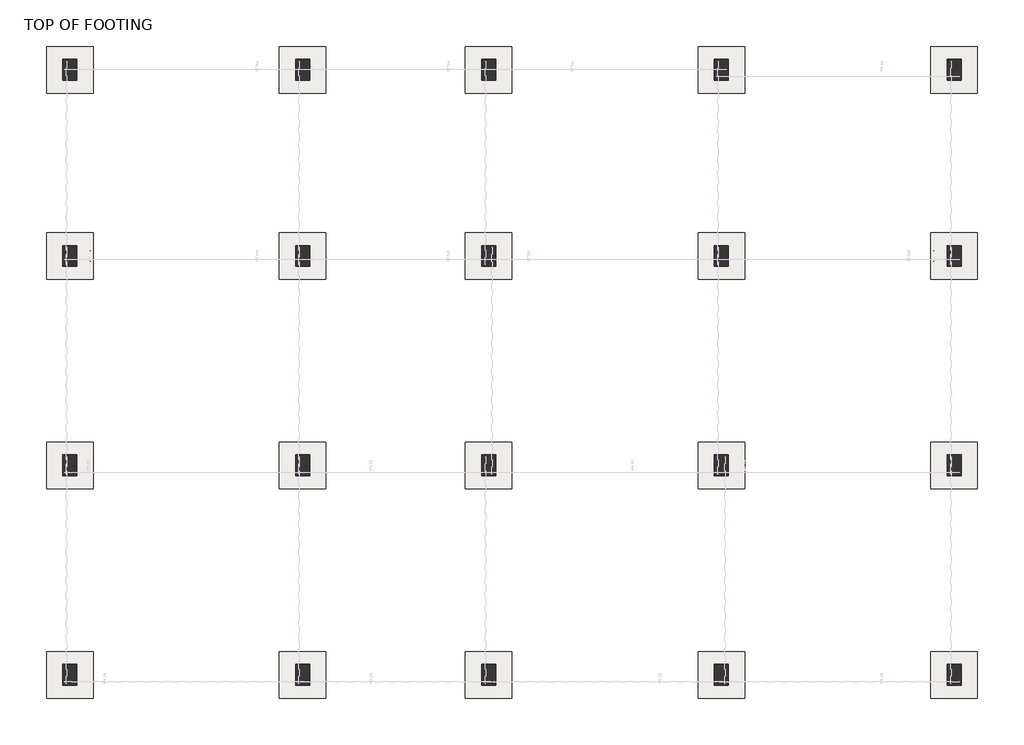
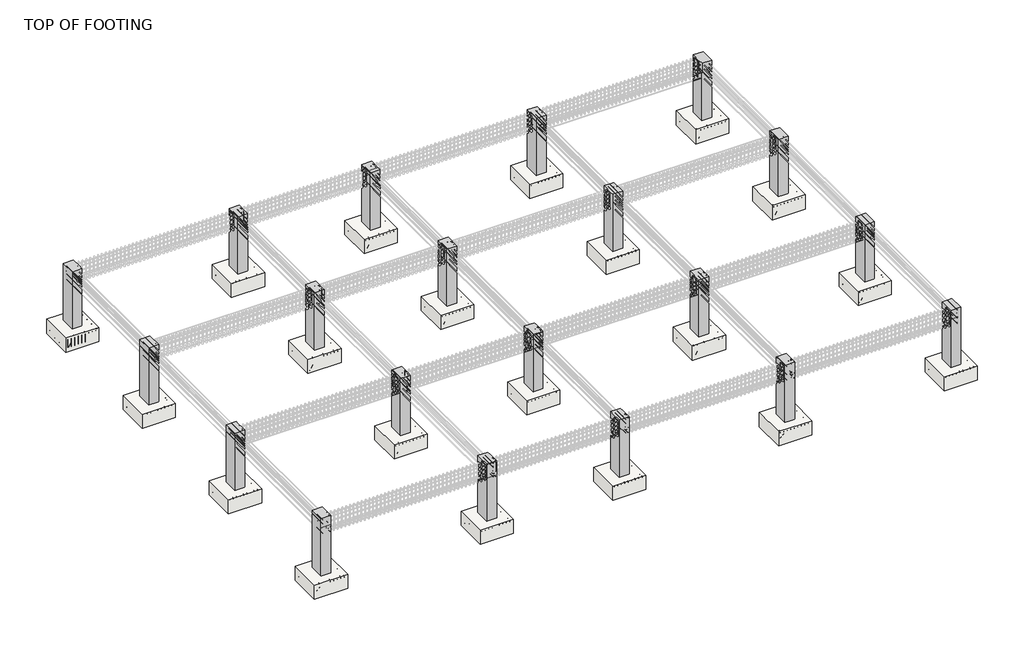
# One storey, part 1 of 13: 20 columns, 20 slabs.
"""IFC4 building model written with IfcOpenShell, lengths in millimetres."""

from ifc_helpers import new_model, si_unit, frame, origin, place, context, project, spatial, polyline, outline, extrude, faceted_brep, transform, mapped, element, save
from components import m_footing_rectangular_4c97ae35

model = new_model("IFC4")

# Units and contexts
model_context = context("Model", 3, world=origin())
ifc_project = project(units=[si_unit("LENGTHUNIT", "METRE", prefix="MILLI")], contexts=[model_context])

# Site, building, storey
site = spatial("IfcSite", under=ifc_project)
building = spatial("IfcBuilding", under=site)
storey = spatial("IfcBuildingStorey", under=building, Name="TOP OF FOOTING", Elevation=-1828.8)

# Columns
placement = place(None, origin())
element("IfcColumn", 1, ObjectType="M_Concrete-Rectangular-Column : 300 x 450mm", at=placement, inside=storey, context=model_context, shape_type="Brep", body=[
    faceted_brep([(-12970.2998378, 16757.5351908, -1828.8), (-12970.2998378, 16307.5351908, -1828.8), (-13270.2998378, 16307.5351908, -1828.8), (-13270.2998378, 16757.5351908, -1828.8), (-12970.2998378, 16757.5351908, 0.0), (-12970.2998378, 16457.5351908, 0.0), (-12970.2998378, 16307.5351908, 0.0), (-13270.2998378, 16307.5351908, 0.0), (-13270.2998378, 16757.5351908, 0.0)], [[[0, 1, 2, 3]], [[4, 5, 6, 1, 0]], [[6, 7, 2, 1]], [[7, 8, 3, 2]], [[8, 4, 0, 3]], [[4, 8, 7, 6, 5]]]),
])
element("IfcColumn", 2, ObjectType="M_Concrete-Rectangular-Column : 300 x 450mm", at=placement, inside=storey, context=model_context, shape_type="Brep", body=[
    faceted_brep([(-7970.2998378, 16757.5351908, -1828.8), (-7970.2998378, 16307.5351908, -1828.8), (-8270.2998378, 16307.5351908, -1828.8), (-8270.2998378, 16757.5351908, -1828.8), (-7970.2998378, 16757.5351908, 0.0), (-7970.2998378, 16457.5351908, 0.0), (-7970.2998378, 16307.5351908, 0.0), (-8270.2998378, 16307.5351908, 0.0), (-8270.2998378, 16457.5351908, 0.0), (-8270.2998378, 16757.5351908, 0.0)], [[[0, 1, 2, 3]], [[4, 5, 6, 1, 0]], [[6, 7, 2, 1]], [[7, 8, 9, 3, 2]], [[9, 4, 0, 3]], [[4, 9, 8, 7, 6, 5]]]),
])
element("IfcColumn", 3, ObjectType="M_Concrete-Rectangular-Column : 300 x 450mm", at=placement, inside=storey, context=model_context, shape_type="Brep", body=[
    faceted_brep([(-3970.2998378, 16757.5351908, -1828.8), (-3970.2998378, 16307.5351908, -1828.8), (-4270.2998378, 16307.5351908, -1828.8), (-4270.2998378, 16757.5351908, -1828.8), (-3970.2998378, 16757.5351908, 0.0), (-3970.2998378, 16461.9874846, 0.0), (-3970.2998378, 16307.5351908, 0.0), (-4270.2998378, 16307.5351908, 0.0), (-4270.2998378, 16457.5351908, 0.0), (-4270.2998378, 16757.5351908, 0.0)], [[[0, 1, 2, 3]], [[4, 5, 6, 1, 0]], [[6, 7, 2, 1]], [[7, 8, 9, 3, 2]], [[9, 4, 0, 3]], [[4, 9, 8, 7, 6, 5]]]),
])
element("IfcColumn", 4, ObjectType="M_Concrete-Rectangular-Column : 300 x 450mm", at=placement, inside=storey, context=model_context, shape_type="SweptSolid", body=[
    extrude(outline(polyline([(1029.7001622, 16757.5351908), (1029.7001622, 16307.5351908), (729.7001622, 16307.5351908), (729.7001622, 16757.5351908), (1029.7001622, 16757.5351908)])), frame((0.0, 0.0, -1828.8), z_axis=(0.0, 0.0, 1.0), x_axis=(1.0, 0.0, 0.0)), (0.0, 0.0, 1.0), 1828.8),
])
element("IfcColumn", 5, ObjectType="M_Concrete-Rectangular-Column : 300 x 450mm", at=placement, inside=storey, context=model_context, shape_type="Brep", body=[
    faceted_brep([(6029.7001622, 16757.5351908, -1828.8), (6029.7001622, 16307.5351908, -1828.8), (5729.7001622, 16307.5351908, -1828.8), (5729.7001622, 16757.5351908, -1828.8), (6029.7001622, 16757.5351908, 0.0), (6029.7001622, 16307.5351908, 0.0), (5735.0295084, 16307.5351908, 0.0), (5735.0295084, 16307.5351908, -300.0), (5729.7001622, 16307.5351908, -300.0), (5729.7001622, 16457.5351908, -300.0), (5729.7001622, 16457.5351908, 0.0), (5729.7001622, 16757.5351908, 0.0), (5735.0295084, 16457.5351908, 0.0), (5735.0295084, 16457.5351908, -300.0)], [[[0, 1, 2, 3]], [[1, 0, 4, 5]], [[2, 1, 5, 6, 7, 8]], [[3, 2, 8, 9, 10, 11]], [[0, 3, 11, 4]], [[5, 4, 11, 10, 12, 6]], [[13, 9, 8, 7]], [[12, 13, 7, 6]], [[13, 12, 10, 9]]]),
])
element("IfcColumn", 6, ObjectType="M_Concrete-Rectangular-Column : 300 x 450mm", at=placement, inside=storey, context=model_context, shape_type="Brep", body=[
    faceted_brep([(6029.7001622, 12757.5351908, -1828.8), (6029.7001622, 12307.5351908, -1828.8), (5729.7001622, 12307.5351908, -1828.8), (5729.7001622, 12757.5351908, -1828.8), (6029.7001622, 12757.5351908, 0.0), (6029.7001622, 12307.5351908, 0.0), (5729.7001622, 12307.5351908, 0.0), (5729.7001622, 12382.5351908, 0.0), (5729.7001622, 12682.5351908, 0.0), (5729.7001622, 12682.5351908, -300.0), (5729.7001622, 12757.5351908, -300.0), (5735.0295084, 12757.5351908, -300.0), (5735.0295084, 12757.5351908, 0.0), (5735.0295084, 12682.5351908, 0.0), (5735.0295084, 12682.5351908, -300.0)], [[[0, 1, 2, 3]], [[1, 0, 4, 5]], [[2, 1, 5, 6]], [[3, 2, 6, 7, 8, 9, 10]], [[0, 3, 10, 11, 12, 4]], [[5, 4, 12, 13, 8, 7, 6]], [[9, 14, 11, 10]], [[14, 13, 12, 11]], [[13, 14, 9, 8]]]),
])
element("IfcColumn", 7, ObjectType="M_Concrete-Rectangular-Column : 300 x 450mm", at=placement, inside=storey, context=model_context, shape_type="Brep", body=[
    faceted_brep([(1029.7001622, 12757.5351908, -1828.8), (1029.7001622, 12307.5351908, -1828.8), (729.7001622, 12307.5351908, -1828.8), (729.7001622, 12757.5351908, -1828.8), (1029.7001622, 12757.5351908, 0.0), (1029.7001622, 12382.5351908, 0.0), (1029.7001622, 12307.5351908, 0.0), (729.7001622, 12307.5351908, 0.0), (729.7001622, 12381.9874846, 0.0), (729.7001622, 12757.5351908, 0.0)], [[[0, 1, 2, 3]], [[4, 5, 6, 1, 0]], [[6, 7, 2, 1]], [[7, 8, 9, 3, 2]], [[9, 4, 0, 3]], [[4, 9, 8, 7, 6, 5]]]),
])
element("IfcColumn", 8, ObjectType="M_Concrete-Rectangular-Column : 300 x 450mm", at=placement, inside=storey, context=model_context, shape_type="Brep", body=[
    faceted_brep([(-3970.2998378, 12757.5351908, -1828.8), (-3970.2998378, 12307.5351908, -1828.8), (-4270.2998378, 12307.5351908, -1828.8), (-4270.2998378, 12757.5351908, -1828.8), (-3970.2998378, 12757.5351908, 0.0), (-3970.2998378, 12682.5351908, 0.0), (-3970.2998378, 12381.9874846, 0.0), (-3970.2998378, 12307.5351908, 0.0), (-4270.2998378, 12307.5351908, 0.0), (-4270.2998378, 12382.5351908, 0.0), (-4270.2998378, 12682.5351908, 0.0), (-4270.2998378, 12757.5351908, 0.0)], [[[0, 1, 2, 3]], [[4, 5, 6, 7, 1, 0]], [[7, 8, 2, 1]], [[8, 9, 10, 11, 3, 2]], [[11, 4, 0, 3]], [[4, 11, 10, 9, 8, 7, 6, 5]]]),
])
element("IfcColumn", 9, ObjectType="M_Concrete-Rectangular-Column : 300 x 450mm", at=placement, inside=storey, context=model_context, shape_type="Brep", body=[
    faceted_brep([(-7970.2998378, 12757.5351908, -1828.8), (-7970.2998378, 12307.5351908, -1828.8), (-8270.2998378, 12307.5351908, -1828.8), (-8270.2998378, 12757.5351908, -1828.8), (-7970.2998378, 12757.5351908, 0.0), (-7970.2998378, 12682.5351908, 0.0), (-7970.2998378, 12382.5351908, 0.0), (-7970.2998378, 12307.5351908, 0.0), (-8270.2998378, 12307.5351908, 0.0), (-8270.2998378, 12382.5351908, 0.0), (-8270.2998378, 12682.5351908, 0.0), (-8270.2998378, 12757.5351908, 0.0)], [[[0, 1, 2, 3]], [[4, 5, 6, 7, 1, 0]], [[7, 8, 2, 1]], [[8, 9, 10, 11, 3, 2]], [[11, 4, 0, 3]], [[4, 11, 10, 9, 8, 7, 6, 5]]]),
])
element("IfcColumn", 10, ObjectType="M_Concrete-Rectangular-Column : 300 x 450mm", at=placement, inside=storey, context=model_context, shape_type="Brep", body=[
    faceted_brep([(-12970.2998378, 12757.5351908, -1828.8), (-12970.2998378, 12307.5351908, -1828.8), (-13270.2998378, 12307.5351908, -1828.8), (-13270.2998378, 12757.5351908, -1828.8), (-12970.2998378, 12757.5351908, 0.0), (-12970.2998378, 12682.5351908, 0.0), (-12970.2998378, 12382.5351908, 0.0), (-12970.2998378, 12307.5351908, 0.0), (-13270.2998378, 12307.5351908, 0.0), (-13270.2998378, 12757.5351908, 0.0)], [[[0, 1, 2, 3]], [[4, 5, 6, 7, 1, 0]], [[7, 8, 2, 1]], [[8, 9, 3, 2]], [[9, 4, 0, 3]], [[4, 9, 8, 7, 6, 5]]]),
])
element("IfcColumn", 11, ObjectType="M_Concrete-Rectangular-Column : 300 x 450mm", at=placement, inside=storey, context=model_context, shape_type="Brep", body=[
    faceted_brep([(-12970.2998378, 8257.5351908, -1828.8), (-12970.2998378, 7807.5351908, -1828.8), (-13270.2998378, 7807.5351908, -1828.8), (-13270.2998378, 8257.5351908, -1828.8), (-12970.2998378, 8257.5351908, 0.0), (-12970.2998378, 8182.5351908, 0.0), (-12970.2998378, 7882.5351908, 0.0), (-12970.2998378, 7807.5351908, 0.0), (-13270.2998378, 7807.5351908, 0.0), (-13270.2998378, 8257.5351908, 0.0)], [[[0, 1, 2, 3]], [[4, 5, 6, 7, 1, 0]], [[7, 8, 2, 1]], [[8, 9, 3, 2]], [[9, 4, 0, 3]], [[4, 9, 8, 7, 6, 5]]]),
])
element("IfcColumn", 12, ObjectType="M_Concrete-Rectangular-Column : 300 x 450mm", at=placement, inside=storey, context=model_context, shape_type="Brep", body=[
    faceted_brep([(-7970.2998378, 8257.5351908, -1828.8), (-7970.2998378, 7807.5351908, -1828.8), (-8270.2998378, 7807.5351908, -1828.8), (-8270.2998378, 8257.5351908, -1828.8), (-7970.2998378, 8257.5351908, 0.0), (-7970.2998378, 8182.5351908, 0.0), (-7970.2998378, 7887.5351908, 0.0), (-7970.2998378, 7807.5351908, 0.0), (-8270.2998378, 7807.5351908, 0.0), (-8270.2998378, 7882.5351908, 0.0), (-8270.2998378, 8182.5351908, 0.0), (-8270.2998378, 8257.5351908, 0.0)], [[[0, 1, 2, 3]], [[4, 5, 6, 7, 1, 0]], [[7, 8, 2, 1]], [[8, 9, 10, 11, 3, 2]], [[11, 4, 0, 3]], [[4, 11, 10, 9, 8, 7, 6, 5]]]),
])
element("IfcColumn", 13, ObjectType="M_Concrete-Rectangular-Column : 300 x 450mm", at=placement, inside=storey, context=model_context, shape_type="Brep", body=[
    faceted_brep([(-3970.2998378, 8257.5351908, -1828.8), (-3970.2998378, 7807.5351908, -1828.8), (-4270.2998378, 7807.5351908, -1828.8), (-4270.2998378, 8257.5351908, -1828.8), (-3970.2998378, 8257.5351908, 0.0), (-3970.2998378, 8182.5351908, 0.0), (-3970.2998378, 7882.5351908, 0.0), (-3970.2998378, 7807.5351908, 0.0), (-4270.2998378, 7807.5351908, 0.0), (-4270.2998378, 7887.5351908, 0.0), (-4270.2998378, 8182.5351908, 0.0), (-4270.2998378, 8257.5351908, 0.0)], [[[0, 1, 2, 3]], [[4, 5, 6, 7, 1, 0]], [[7, 8, 2, 1]], [[8, 9, 10, 11, 3, 2]], [[11, 4, 0, 3]], [[4, 11, 10, 9, 8, 7, 6, 5]]]),
])
element("IfcColumn", 14, ObjectType="M_Concrete-Rectangular-Column : 300 x 450mm", at=placement, inside=storey, context=model_context, shape_type="Brep", body=[
    faceted_brep([(1029.7001622, 8257.5351908, -1828.8), (1029.7001622, 7807.5351908, -1828.8), (729.7001622, 7807.5351908, -1828.8), (729.7001622, 8257.5351908, -1828.8), (1029.7001622, 8257.5351908, 0.0), (1029.7001622, 8182.5351908, 0.0), (1029.7001622, 7882.5351908, 0.0), (1029.7001622, 7807.5351908, 0.0), (729.7001622, 7807.5351908, 0.0), (729.7001622, 7882.5351908, 0.0), (729.7001622, 8182.5351908, 0.0), (729.7001622, 8257.5351908, 0.0)], [[[0, 1, 2, 3]], [[4, 5, 6, 7, 1, 0]], [[7, 8, 2, 1]], [[8, 9, 10, 11, 3, 2]], [[11, 4, 0, 3]], [[4, 11, 10, 9, 8, 7, 6, 5]]]),
])
element("IfcColumn", 15, ObjectType="M_Concrete-Rectangular-Column : 300 x 450mm", at=placement, inside=storey, context=model_context, shape_type="Brep", body=[
    faceted_brep([(6029.7001622, 8257.5351908, -1828.8), (6029.7001622, 7807.5351908, -1828.8), (5729.7001622, 7807.5351908, -1828.8), (5729.7001622, 8257.5351908, -1828.8), (6029.7001622, 8257.5351908, 0.0), (6029.7001622, 7807.5351908, 0.0), (5729.7001622, 7807.5351908, 0.0), (5729.7001622, 7882.5351908, 0.0), (5729.7001622, 8182.5351908, 0.0), (5729.7001622, 8257.5351908, 0.0)], [[[0, 1, 2, 3]], [[4, 5, 1, 0]], [[5, 6, 2, 1]], [[6, 7, 8, 9, 3, 2]], [[9, 4, 0, 3]], [[4, 9, 8, 7, 6, 5]]]),
])
element("IfcColumn", 16, ObjectType="M_Concrete-Rectangular-Column : 300 x 450mm", at=placement, inside=storey, context=model_context, shape_type="Brep", body=[
    faceted_brep([(-12970.2998378, 3757.5351908, -1828.8), (-12970.2998378, 3307.5351908, -1828.8), (-13270.2998378, 3307.5351908, -1828.8), (-13270.2998378, 3757.5351908, -1828.8), (-12970.2998378, 3757.5351908, 0.0), (-12970.2998378, 3607.5351908, 0.0), (-12970.2998378, 3307.5351908, 0.0), (-13270.2998378, 3307.5351908, 0.0), (-13270.2998378, 3757.5351908, 0.0)], [[[0, 1, 2, 3]], [[4, 5, 6, 1, 0]], [[6, 7, 2, 1]], [[7, 8, 3, 2]], [[8, 4, 0, 3]], [[4, 8, 7, 6, 5]]]),
])
element("IfcColumn", 17, ObjectType="M_Concrete-Rectangular-Column : 300 x 450mm", at=placement, inside=storey, context=model_context, shape_type="Brep", body=[
    faceted_brep([(-7970.2998378, 3757.5351908, -1828.8), (-7970.2998378, 3307.5351908, -1828.8), (-8270.2998378, 3307.5351908, -1828.8), (-8270.2998378, 3757.5351908, -1828.8), (-7970.2998378, 3757.5351908, 0.0), (-7970.2998378, 3607.5351908, 0.0), (-7970.2998378, 3307.5351908, 0.0), (-8270.2998378, 3307.5351908, 0.0), (-8270.2998378, 3607.5351908, 0.0), (-8270.2998378, 3757.5351908, 0.0)], [[[0, 1, 2, 3]], [[4, 5, 6, 1, 0]], [[6, 7, 2, 1]], [[7, 8, 9, 3, 2]], [[9, 4, 0, 3]], [[4, 9, 8, 7, 6, 5]]]),
])
element("IfcColumn", 18, ObjectType="M_Concrete-Rectangular-Column : 300 x 450mm", at=placement, inside=storey, context=model_context, shape_type="Brep", body=[
    faceted_brep([(-3970.2998378, 3757.5351908, -1828.8), (-3970.2998378, 3307.5351908, -1828.8), (-4270.2998378, 3307.5351908, -1828.8), (-4270.2998378, 3757.5351908, -1828.8), (-3970.2998378, 3757.5351908, 0.0), (-3970.2998378, 3607.5351908, 0.0), (-3970.2998378, 3307.5351908, 0.0), (-4270.2998378, 3307.5351908, 0.0), (-4270.2998378, 3607.5351908, 0.0), (-4270.2998378, 3757.5351908, 0.0)], [[[0, 1, 2, 3]], [[4, 5, 6, 1, 0]], [[6, 7, 2, 1]], [[7, 8, 9, 3, 2]], [[9, 4, 0, 3]], [[4, 9, 8, 7, 6, 5]]]),
])
element("IfcColumn", 19, ObjectType="M_Concrete-Rectangular-Column : 300 x 450mm", at=placement, inside=storey, context=model_context, shape_type="Brep", body=[
    faceted_brep([(1029.7001622, 3757.5351908, -1828.8), (1029.7001622, 3307.5351908, -1828.8), (729.7001622, 3307.5351908, -1828.8), (729.7001622, 3757.5351908, -1828.8), (1029.7001622, 3757.5351908, 0.0), (1029.7001622, 3607.5351908, 0.0), (1029.7001622, 3307.5351908, 0.0), (729.7001622, 3307.5351908, 0.0), (729.7001622, 3607.5351908, 0.0), (729.7001622, 3757.5351908, 0.0)], [[[0, 1, 2, 3]], [[4, 5, 6, 1, 0]], [[6, 7, 2, 1]], [[7, 8, 9, 3, 2]], [[9, 4, 0, 3]], [[4, 9, 8, 7, 6, 5]]]),
])
element("IfcColumn", 20, ObjectType="M_Concrete-Rectangular-Column : 300 x 450mm", at=placement, inside=storey, context=model_context, shape_type="Brep", body=[
    faceted_brep([(6029.7001622, 3757.5351908, -1828.8), (6029.7001622, 3307.5351908, -1828.8), (5729.7001622, 3307.5351908, -1828.8), (5729.7001622, 3757.5351908, -1828.8), (6029.7001622, 3757.5351908, 0.0), (6029.7001622, 3307.5351908, 0.0), (5729.7001622, 3307.5351908, 0.0), (5729.7001622, 3607.5351908, 0.0), (5729.7001622, 3757.5351908, 0.0)], [[[0, 1, 2, 3]], [[4, 5, 1, 0]], [[5, 6, 2, 1]], [[6, 7, 8, 3, 2]], [[8, 4, 0, 3]], [[4, 8, 7, 6, 5]]]),
])

# Slabs
m_footing_rectangular_shape = m_footing_rectangular_4c97ae35(model_context)
element("IfcSlab", 21, ObjectType="M_Footing-Rectangular", at=placement, inside=storey, context=model_context, shape_type="MappedRepresentation", body=[
    mapped(m_footing_rectangular_shape, transform((-13120.2998378, 16532.5351908, -1828.8), x_axis=(1.0, 0.0, 0.0), y_axis=(0.0, 1.0, 0.0), z_axis=(0.0, 0.0, 1.0))),
])
element("IfcSlab", 22, ObjectType="M_Footing-Rectangular", at=placement, inside=storey, context=model_context, shape_type="MappedRepresentation", body=[
    mapped(m_footing_rectangular_shape, transform((-8120.2998378, 16532.5351908, -1828.8), x_axis=(1.0, 0.0, 0.0), y_axis=(0.0, 1.0, 0.0), z_axis=(0.0, 0.0, 1.0))),
])
element("IfcSlab", 23, ObjectType="M_Footing-Rectangular", at=placement, inside=storey, context=model_context, shape_type="MappedRepresentation", body=[
    mapped(m_footing_rectangular_shape, transform((-4120.2998378, 16532.5351908, -1828.8), x_axis=(1.0, 0.0, 0.0), y_axis=(0.0, 1.0, 0.0), z_axis=(0.0, 0.0, 1.0))),
])
element("IfcSlab", 24, ObjectType="M_Footing-Rectangular", at=placement, inside=storey, context=model_context, shape_type="MappedRepresentation", body=[
    mapped(m_footing_rectangular_shape, transform((879.7001622, 16532.5351908, -1828.8), x_axis=(1.0, 0.0, 0.0), y_axis=(0.0, 1.0, 0.0), z_axis=(0.0, 0.0, 1.0))),
])
element("IfcSlab", 25, ObjectType="M_Footing-Rectangular", at=placement, inside=storey, context=model_context, shape_type="MappedRepresentation", body=[
    mapped(m_footing_rectangular_shape, transform((5879.7001622, 16532.5351908, -1828.8), x_axis=(1.0, 0.0, 0.0), y_axis=(0.0, 1.0, 0.0), z_axis=(0.0, 0.0, 1.0))),
])
element("IfcSlab", 26, ObjectType="M_Footing-Rectangular", at=placement, inside=storey, context=model_context, shape_type="MappedRepresentation", body=[
    mapped(m_footing_rectangular_shape, transform((5879.7001622, 12532.5351908, -1828.8), x_axis=(1.0, 0.0, 0.0), y_axis=(0.0, 1.0, 0.0), z_axis=(0.0, 0.0, 1.0))),
])
element("IfcSlab", 27, ObjectType="M_Footing-Rectangular", at=placement, inside=storey, context=model_context, shape_type="MappedRepresentation", body=[
    mapped(m_footing_rectangular_shape, transform((879.7001622, 12532.5351908, -1828.8), x_axis=(1.0, 0.0, 0.0), y_axis=(0.0, 1.0, 0.0), z_axis=(0.0, 0.0, 1.0))),
])
element("IfcSlab", 28, ObjectType="M_Footing-Rectangular", at=placement, inside=storey, context=model_context, shape_type="MappedRepresentation", body=[
    mapped(m_footing_rectangular_shape, transform((-4120.2998378, 12532.5351908, -1828.8), x_axis=(1.0, 0.0, 0.0), y_axis=(0.0, 1.0, 0.0), z_axis=(0.0, 0.0, 1.0))),
])
element("IfcSlab", 29, ObjectType="M_Footing-Rectangular", at=placement, inside=storey, context=model_context, shape_type="MappedRepresentation", body=[
    mapped(m_footing_rectangular_shape, transform((-8120.2998378, 12532.5351908, -1828.8), x_axis=(1.0, 0.0, 0.0), y_axis=(0.0, 1.0, 0.0), z_axis=(0.0, 0.0, 1.0))),
])
element("IfcSlab", 30, ObjectType="M_Footing-Rectangular", at=placement, inside=storey, context=model_context, shape_type="MappedRepresentation", body=[
    mapped(m_footing_rectangular_shape, transform((-13120.2998378, 12532.5351908, -1828.8), x_axis=(1.0, 0.0, 0.0), y_axis=(0.0, 1.0, 0.0), z_axis=(0.0, 0.0, 1.0))),
])
element("IfcSlab", 31, ObjectType="M_Footing-Rectangular", at=placement, inside=storey, context=model_context, shape_type="MappedRepresentation", body=[
    mapped(m_footing_rectangular_shape, transform((-13120.2998378, 8032.5351908, -1828.8), x_axis=(1.0, 0.0, 0.0), y_axis=(0.0, 1.0, 0.0), z_axis=(0.0, 0.0, 1.0))),
])
element("IfcSlab", 32, ObjectType="M_Footing-Rectangular", at=placement, inside=storey, context=model_context, shape_type="MappedRepresentation", body=[
    mapped(m_footing_rectangular_shape, transform((-8120.2998378, 8032.5351908, -1828.8), x_axis=(1.0, 0.0, 0.0), y_axis=(0.0, 1.0, 0.0), z_axis=(0.0, 0.0, 1.0))),
])
element("IfcSlab", 33, ObjectType="M_Footing-Rectangular", at=placement, inside=storey, context=model_context, shape_type="MappedRepresentation", body=[
    mapped(m_footing_rectangular_shape, transform((-4120.2998378, 8032.5351908, -1828.8), x_axis=(1.0, 0.0, 0.0), y_axis=(0.0, 1.0, 0.0), z_axis=(0.0, 0.0, 1.0))),
])
element("IfcSlab", 34, ObjectType="M_Footing-Rectangular", at=placement, inside=storey, context=model_context, shape_type="MappedRepresentation", body=[
    mapped(m_footing_rectangular_shape, transform((879.7001622, 8032.5351908, -1828.8), x_axis=(1.0, 0.0, 0.0), y_axis=(0.0, 1.0, 0.0), z_axis=(0.0, 0.0, 1.0))),
])
element("IfcSlab", 35, ObjectType="M_Footing-Rectangular", at=placement, inside=storey, context=model_context, shape_type="MappedRepresentation", body=[
    mapped(m_footing_rectangular_shape, transform((5879.7001622, 8032.5351908, -1828.8), x_axis=(1.0, 0.0, 0.0), y_axis=(0.0, 1.0, 0.0), z_axis=(0.0, 0.0, 1.0))),
])
element("IfcSlab", 36, ObjectType="M_Footing-Rectangular", at=placement, inside=storey, context=model_context, shape_type="MappedRepresentation", body=[
    mapped(m_footing_rectangular_shape, transform((5879.7001622, 3532.5351908, -1828.8), x_axis=(1.0, 0.0, 0.0), y_axis=(0.0, 1.0, 0.0), z_axis=(0.0, 0.0, 1.0))),
])
element("IfcSlab", 37, ObjectType="M_Footing-Rectangular", at=placement, inside=storey, context=model_context, shape_type="MappedRepresentation", body=[
    mapped(m_footing_rectangular_shape, transform((879.7001622, 3532.5351908, -1828.8), x_axis=(1.0, 0.0, 0.0), y_axis=(0.0, 1.0, 0.0), z_axis=(0.0, 0.0, 1.0))),
])
element("IfcSlab", 38, ObjectType="M_Footing-Rectangular", at=placement, inside=storey, context=model_context, shape_type="MappedRepresentation", body=[
    mapped(m_footing_rectangular_shape, transform((-4120.2998378, 3532.5351908, -1828.8), x_axis=(1.0, 0.0, 0.0), y_axis=(0.0, 1.0, 0.0), z_axis=(0.0, 0.0, 1.0))),
])
element("IfcSlab", 39, ObjectType="M_Footing-Rectangular", at=placement, inside=storey, context=model_context, shape_type="MappedRepresentation", body=[
    mapped(m_footing_rectangular_shape, transform((-8120.2998378, 3532.5351908, -1828.8), x_axis=(1.0, 0.0, 0.0), y_axis=(0.0, 1.0, 0.0), z_axis=(0.0, 0.0, 1.0))),
])
element("IfcSlab", 40, ObjectType="M_Footing-Rectangular", at=placement, inside=storey, context=model_context, shape_type="MappedRepresentation", body=[
    mapped(m_footing_rectangular_shape, transform((-13120.2998378, 3532.5351908, -1828.8), x_axis=(1.0, 0.0, 0.0), y_axis=(0.0, 1.0, 0.0), z_axis=(0.0, 0.0, 1.0))),
])

save(model, "model.ifc")

# Revit data of these elements
# Grids (mm)
#   "1": line (-13120.3, 19861.839) -> (-13120.3, -12631.901)
#   "2": line (-8120.3, 19861.839) -> (-8120.3, -12631.901)
#   "3": line (-4120.3, 19861.839) -> (-4120.3, -12631.901)
#   "4": line (879.7, 19861.839) -> (879.7, -12631.901)
#   "5": line (5879.7, 19861.839) -> (5879.7, -12631.901)
#   "A": line (8041.345, 16532.535) -> (-17991.754, 16532.535)
#   "B": line (8041.345, 12532.535) -> (-17991.754, 12532.535)
#   "C": line (8041.345, 8032.535) -> (-17991.754, 8032.535)
#   "D": line (8041.345, 3532.535) -> (-17991.754, 3532.535)
# Type "M_Concrete-Rectangular-Column : 300 x 450mm"
#   b = 300 mm
#   h = 450 mm
#   Structural Material [instance default] = Concrete, Cast-in-Place gray
# Type "M_Footing-Rectangular"
#   Width = 1000 mm
#   Length = 1000 mm
#   Foundation Thickness = 450 mm
#   Structural Material [instance default] = Concrete, Cast-in-Place gray
#   Assembly Code = ""
# Elements 1, 2, 3, 4, 5, 6, 7, 8, 9, 10, 11, 12, 13, 14, 15, 16, 17, 18, 19, 20 (IfcColumn, "M_Concrete-Rectangular-Column : 300 x 450mm")
#   Structural Material = Concrete, Cast-in-Place gray
#   Phase Created = New Construction
#   Materials on its faces: "Concrete, Cast-in-Place gray"
# Elements 21, 22, 23, 24, 25, 26, 27, 28, 29, 30, 31, 32, 33, 34, 35, 36, 37, 38, 39, 40 (IfcSlab, "M_Footing-Rectangular")
#   Structural Material = Concrete, Cast-in-Place gray
#   Phase Created = New Construction
#   Materials on its faces: "Concrete, Cast-in-Place gray"
# Materials
#   "Concrete, Cast-in-Place gray": class "Concrete", colour RGB 192 192 192, transparency 0, Description = "Cast-in-place concrete", Cost = 0
